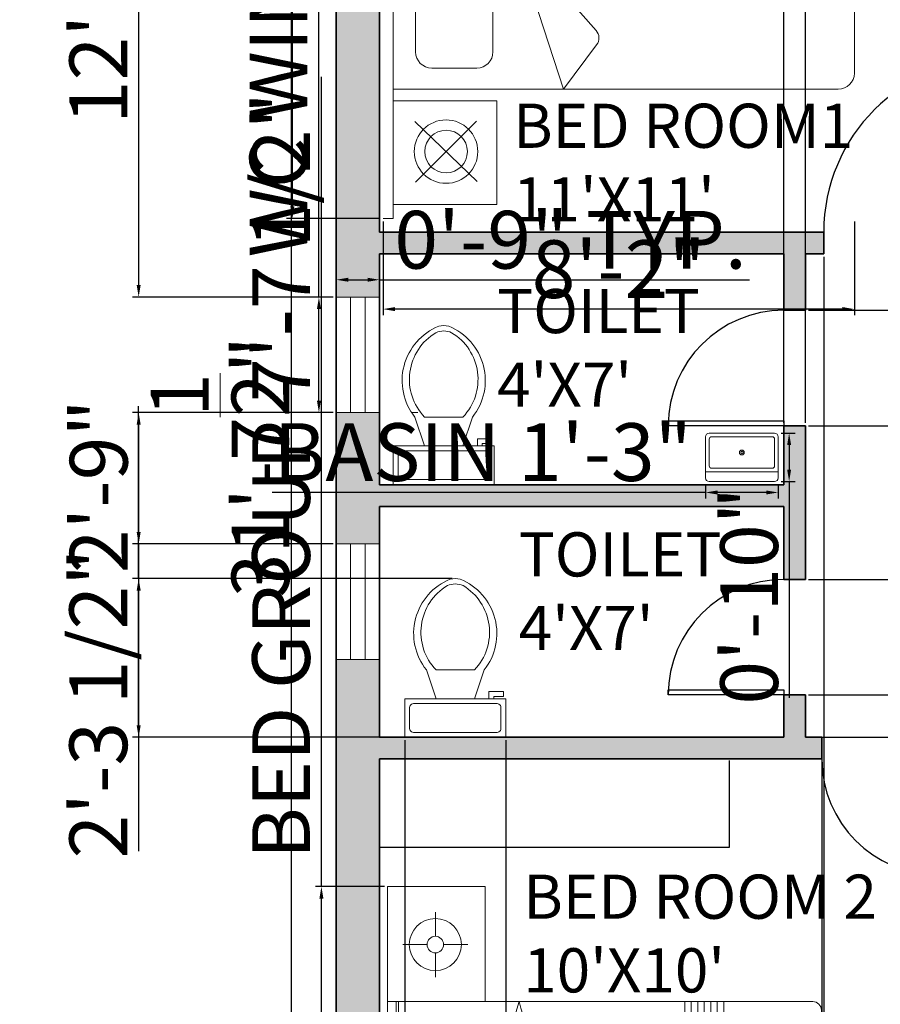
# Model space of a CAD drawing. Units: inches. Extents: x 1810 to 2254, y 313 to 1026.
# Tile 3 of 7: x 1810 to 1988, y 559 to 764. Entities that reach past the tile are written whole.
import ezdxf

# ---------------------------------------------------------------- set-up
doc = ezdxf.new("R2010")
doc.units = ezdxf.units.IN
for name, color, linetype, lineweight in [('A-ANNO-DIMS', 2, 'Continuous', 18), ('A-AREA-IDEN', 7, 'Continuous', 25), ('A-DOOR', 4, 'Continuous', 25), ('A-FLOR-CASE', 8, 'Continuous', 25), ('A-FLOR-FIXT', 9, 'Continuous', 18), ('A-FURN', 8, 'Continuous', 18), ('A-GLAZ', 4, 'Continuous', 18), ('A-WALL', 7, 'Continuous', 35)]:
    doc.layers.add(name, color=color, linetype=linetype, lineweight=lineweight)
doc.layers.add('A-WALL-PATT', color=252, linetype='Continuous', lineweight=13, true_color=0x939598)
doc.styles.add('ATTR', font='romans.shx', dxfattribs={"width": 0.8, "height": 1.075})
doc.styles.get("Standard").update_dxf_attribs({"font": 'arial.ttf'})
doc.dimstyles.new('ISO-25', dxfattribs={"dimtxt": 12, "dimasz": 2.5, "dimexe": 1.25, "dimexo": 0.625, "dimtad": 1, "dimdec": 1, "dimlunit": 4, "dimtxsty": 'Standard', "dimcen": 2.5, "dimadec": 0, "dimazin": 0, "dimtfac": 1, "dimtdec": 1, "dimtmove": 0, "dimatfit": 3, "dimfxl": 1, "dimarcsym": 0})

# ---------------------------------------------------------------- blocks, each defined once
blk = doc.blocks.new('A$C5C1F5B49')
for p, q in [((0, 2), (0, 2.0434)), ((2.6204, 1.9984), (2.6204, 2.0434)), ((0, 2), (2.6204, 2)), ((0.5102, 2), (0.0602, 2)), ((0.0602, 2), (0.0602, 1.55)), ((0.5102, 1.55), (0.5102, 2)), ((0.5602, 2), (0.5602, 0.07)), ((2.0602, 2), (0.5602, 2)), ((2.0602, 0.07), (2.0602, 2)), ((2.5602, 2), (2.1102, 2)), ((2.1102, 2), (2.1102, 1.55)), ((2.5602, 1.55), (2.5602, 2)), ((0.1574, 1.9028), (0.4225, 1.6377)), ((0.1602, 1.635), (0.4197, 1.9056)), ((1.2033, 1.9024), (0.7221, 1.9024)), ((1.919, 1.9024), (1.4378, 1.9024)), ((2.2074, 1.9028), (2.4725, 1.6377)), ((2.2102, 1.635), (2.4697, 1.9056)), ((0.6521, 1.8324), (0.6521, 1.6369)), ((1.2733, 1.6369), (1.2733, 1.8324)), ((1.3678, 1.8324), (1.3678, 1.6369)), ((1.989, 1.6369), (1.989, 1.8324)), ((0.0602, 1.55), (0.5102, 1.55)), ((0.7221, 1.5669), (1.2033, 1.5669)), ((1.4378, 1.5669), (1.919, 1.5669)), ((2.1102, 1.55), (2.5602, 1.55)), ((0.5602, 1.2611), (1.2132, 1.4737)), ((1.2066, 1.4637), (0.8154, 1.12)), ((1.3997, 1.4761), (1.2396, 1.4761)), ((1.3997, 1.4761), (1.805, 1.12)), ((2.0602, 1.2611), (1.3997, 1.4761)), ((0.7525, 1.1175), (0.5602, 1.2611)), ((1.868, 1.1175), (2.0602, 1.2611)), ((0.6302, 0), (1.9902, 0))]:
    blk.add_line(p, q)
for centre, radius in [((0.2899, 1.7703), 0.1375), ((2.3399, 1.7703), 0.1375), ((0.2899, 1.7703), 0.0925), ((2.3399, 1.7703), 0.0925)]:
    blk.add_circle(centre, radius)
for centre, radius, start, end in [((0.7221, 1.8324), 0.07, 90, 180), ((1.2033, 1.8324), 0.07, 0, 90), ((1.4378, 1.8324), 0.07, 90, 180), ((1.919, 1.8324), 0.07, 0, 90), ((0.7221, 1.6369), 0.07, 180, 270), ((1.2033, 1.6369), 0.07, 270, 0), ((1.4378, 1.6369), 0.07, 180, 270), ((1.919, 1.6369), 0.07, 270, 0), ((1.2396, 1.4261), 0.05, 90, 131.3042), ((1.2287, 1.4261), 0.05, 90, 108.034), ((0.7824, 1.1575), 0.05, 233.2421, 311.3042), ((1.838, 1.1575), 0.05, 228.6958, 306.7579), ((0.6302, 0.07), 0.07, 180, 270), ((1.9902, 0.07), 0.07, 270, 0)]:
    blk.add_arc(centre, radius, start, end)
blk = doc.blocks.new('A$C50CC761E')
for p, q in [((0, 2), (0, 0.04)), ((0, 2), (1.5, 2)), ((1.5, 2), (1.5, 0.04)), ((0, 1.96), (1.5, 1.96)), ((0, 1.95), (1.5, 1.95)), ((0, 0.63), (1.5, 0.63)), ((0, 0.6), (1.5, 0.6)), ((0, 0.57), (1.5, 0.57)), ((0, 0.54), (1.5, 0.54)), ((0, 0.51), (1.5, 0.51)), ((0, 0.48), (1.5, 0.48)), ((0, 0.45), (1.5, 0.45)), ((1.46, 0), (0.04, 0))]:
    blk.add_line(p, q)
at = {"ltscale": 250}
for p, q in [((1.5, 2), (2.0303, 2)), ((2.0303, 2), (2.0303, 1.5501)), ((1.763, 1.8176), (1.763, 1.9295)), ((1.613, 1.7795), (1.7249, 1.7795)), ((1.8011, 1.7795), (1.913, 1.7795)), ((1.763, 1.6295), (1.763, 1.7414)), ((1.5, 1.5501), (2.0303, 1.5501))]:
    blk.add_line(p, q, dxfattribs=at)
for radius in [0.12, 0.0381]:
    blk.add_circle((1.763, 1.7795), radius, dxfattribs=at)
for centre, radius, start, end in [((0.3894, 5.1577), 3.2899, 265.4501, 274.5499), ((-0.4158, 1.744), 0.5605, 346.15, 13.85), ((0.1321, 1.5916), 0.3789, 4.7708, 46.8165), ((0.1321, 1.5916), 0.4089, 4.1373, 42.5614), ((0.1321, 1.5916), 0.4389, 3.5318, 39.1874), ((0.1321, 1.5916), 0.4689, 2.9489, 36.4321), ((1.1324, 1.744), 0.5004, 164.4468, 195.5532), ((1.1357, 5.1577), 3.2899, 265.4501, 274.5499), ((0.3306, 1.744), 0.5605, 346.15, 13.85), ((0.8784, 1.5916), 0.3789, 4.7708, 46.8165), ((0.8784, 1.5916), 0.4089, 4.1373, 42.5614), ((0.8784, 1.5916), 0.4389, 3.5318, 39.1874), ((0.8784, 1.5916), 0.4689, 2.9489, 36.4321), ((1.8788, 1.744), 0.5004, 164.4468, 195.5532), ((0.3894, -0.4129), 2.0395, 82.6483, 97.3517), ((1.1357, -0.4129), 2.0395, 82.6483, 97.3517), ((1.0573, -0.0269), 1.4879, 72.6898, 135.2822), ((1.6044, 0.9359), 0.4695, 102.8515, 161.769), ((0.6316, 0.0846), 1.1287, 62.1724, 124.0295), ((0.04, 0.04), 0.04, 180, 270), ((1.46, 0.04), 0.04, 270, 0)]:
    blk.add_arc(centre, radius, start, end)
blk = doc.blocks.new('*U4')
for p, q in [((9.5, -6), (9.5, -2)), ((-8, -8.5), (-8, -8)), ((-7, -8), (-7, -9.5)), ((-4, -8), (-6, -14)), ((4, -8), (6, -14)), ((-10, -8.5), (-8, -8.5)), ((-10, -9.5), (-10, -8.5)), ((-7, -9.5), (-10, -9.5)), ((4, -14), (-4, -14))]:
    blk.add_line(p, q)
blk.add_lwpolyline([(10.5, -8), (10.5, 0), (-10.5, 0), (-10.5, -8)], close=True)
for points in [[(-9.5, -2), (-9.5, -6)], [(8.5, -1), (-8.5, -1)], [(-8.5, -7), (8.5, -7)]]:
    blk.add_lwpolyline(points)
for centre, radius, start, end in [((-8.62, -1.88), 0.884, 81.8699, 188.1301), ((8.62, -1.88), 0.884, 351.8699, 98.1301), ((-8.62, -6.12), 0.884, 171.8699, 278.1301), ((8.62, -6.12), 0.884, 261.8699, 8.1301), ((3.52, -21.58), 12.17, 141.4691, 247.9714), ((4.2, -21.82), 11.33, 136.3677, 238.9468), ((-3.52, -21.58), 12.17, 292.0284, 38.5307), ((-4.2, -21.82), 11.33, 301.053, 43.6321), ((0, -27.88), 4, 245.7318, 294.2682), ((0, -29), 4, 254.8605, 285.1395)]:
    blk.add_arc(centre, radius, start, end)
blk = doc.blocks.new("30'' Sink Single PV")
blk.add_line((-15, -3.999996), (15, -3.999996))
for points in [[(-13.5, 0), (13.5, 0)], [(-15, -18.499996), (-15, -1.5)], [(15, -1.5), (15, -18.499996)], [(-13.5, -17.499996), (-13.5, -6.499996)], [(-12.5, -5.499996), (12.5, -5.499996)], [(13.5, -6.499996), (13.5, -17.499996)], [(13.5, -19.999996), (-13.5, -19.999996)], [(12.5, -18.499996), (-12.5, -18.499996)]]:
    blk.add_lwpolyline(points)
for radius in [1, 0.5]:
    blk.add_circle((0, -11.999996), radius)
for centre, radius, start, end in [((-13.5, -1.5), 1.5, 90, 180), ((13.5, -1.5), 1.5, 0, 90), ((-12.5, -6.499996), 1, 90, 180), ((12.5, -6.499996), 1, 0, 90), ((-13.5, -18.499996), 1.5, 180, 270), ((-12.5, -17.499996), 1, 180, 270), ((12.5, -17.499996), 1, 270, 0), ((13.5, -18.499996), 1.5, 270, 0)]:
    blk.add_arc(centre, radius, start, end)
at = {"style": 'ATTR', "width": 0.8, "flags": 9}
blk.add_attdef('ESTCODE', (0, 0), '', height=0.006, dxfattribs=at)
blk = doc.blocks.new('*U17')
for p, q in [((0, 0), (0, -4)), ((-40, 0), (-40, -4))]:
    blk.add_line(p, q)
blk.add_lwpolyline([(0, 0), (0, 40), (-1.75, 40), (-1.75, 0)], close=True)
blk.add_arc((0, 0), 40, 90, 180)
blk = doc.blocks.new('*U16')
for p, q in [((0, 0), (0, -6)), ((40, 0), (40, -6))]:
    blk.add_line(p, q)
blk.add_lwpolyline([(0, 0), (0, 40), (1.75, 40), (1.75, 0)], close=True)
blk.add_arc((0, 0), 40, 0, 90)
blk = doc.blocks.new('*D25')
at = {"layer": 'A-ANNO-DIMS', "color": 0, "lineweight": -2, "transparency": 16777216}
for p, q in [((1874.74, 860.61), (1864.75, 860.61)), ((1866, 858.11), (1866, 483.61)), ((1874.74, 481.11), (1864.75, 481.11))]:
    blk.add_line(p, q, dxfattribs=at)
at = {"layer": 'A-ANNO-DIMS', "color": 0, "transparency": 16777216}
for points in [[(1865.58, 858.11), (1866.42, 858.11), (1866, 860.61)], [(1865.58, 483.61), (1866.42, 483.61), (1866, 481.11)]]:
    blk.add_solid(points, dxfattribs=at)
at = {"layer": 'Defpoints', "color": 0, "transparency": 16777216}
for p in [(1875.36, 860.61), (1866, 481.11), (1875.36, 481.11)]:
    blk.add_point(p, dxfattribs=at)
at = {"layer": 'A-ANNO-DIMS', "color": 0, "transparency": 16777216, "insert": (1851.22, 670.86), "char_height": 12, "attachment_point": 5, "rotation": 90}
blk.add_mtext('31\'-7{\\H1x;\\S1/2;}"', dxfattribs=at)
blk = doc.blocks.new('WIN-24IN-WALL9')
for p, q in [((9, 24), (0, 24)), ((3, 24), (3, 0)), ((6, 24), (6, 0)), ((9, 0), (0, 0))]:
    blk.add_line(p, q)
blk = doc.blocks.new('*D34')
at = {"layer": 'A-ANNO-DIMS', "color": 0, "lineweight": -2, "transparency": 16777216}
for p, q in [((1871.76, 706.11), (1871.76, 894.3)), ((1874.74, 706.11), (1870.51, 706.11)), ((1871.76, 684.61), (1871.76, 703.61)), ((1874.74, 682.11), (1870.51, 682.11))]:
    blk.add_line(p, q, dxfattribs=at)
at = {"layer": 'A-ANNO-DIMS', "color": 0, "transparency": 16777216}
for points in [[(1871.35, 703.61), (1872.18, 703.61), (1871.76, 706.11)], [(1871.35, 684.61), (1872.18, 684.61), (1871.76, 682.11)]]:
    blk.add_solid(points, dxfattribs=at)
at = {"layer": 'Defpoints', "color": 0, "transparency": 16777216}
for p in [(1871.76, 706.11), (1875.36, 706.11), (1875.36, 682.11)]:
    blk.add_point(p, dxfattribs=at)
at = {"layer": 'A-ANNO-DIMS', "color": 0, "transparency": 16777216, "insert": (1864.93, 801.46), "char_height": 12, "attachment_point": 5, "rotation": 90}
blk.add_mtext('WC WINDOW 2\'-0" TYP.', dxfattribs=at)
blk = doc.blocks.new('*D35')
at = {"layer": 'A-ANNO-DIMS', "color": 0, "lineweight": -2, "transparency": 16777216}
for p, q in [((1875.36, 706.74), (1875.36, 710.96)), ((1884.36, 706.74), (1884.36, 710.96)), ((1877.86, 709.71), (1881.86, 709.71)), ((1884.36, 709.71), (1961.26, 709.71))]:
    blk.add_line(p, q, dxfattribs=at)
at = {"layer": 'A-ANNO-DIMS', "color": 0, "transparency": 16777216}
for points in [[(1877.86, 710.13), (1877.86, 709.3), (1875.36, 709.71)], [(1881.86, 710.13), (1881.86, 709.3), (1884.36, 709.71)]]:
    blk.add_solid(points, dxfattribs=at)
at = {"layer": 'Defpoints', "color": 0, "transparency": 16777216}
for p in [(1884.36, 709.71), (1875.36, 706.11), (1884.36, 706.11)]:
    blk.add_point(p, dxfattribs=at)
at = {"layer": 'A-ANNO-DIMS', "color": 0, "transparency": 16777216, "insert": (1924.06, 716.47), "char_height": 12, "attachment_point": 5}
blk.add_mtext('0\'-9" TYP.', dxfattribs=at)
blk = doc.blocks.new('*D36')
at = {"layer": 'A-ANNO-DIMS', "color": 0, "lineweight": -2, "transparency": 16777216}
for p, q in [((1866.25, 848.07), (1866.25, 1025.73)), ((1884.47, 848.07), (1865, 848.07)), ((1866.25, 724.95), (1866.25, 845.57)), ((1884.47, 722.45), (1865, 722.45))]:
    blk.add_line(p, q, dxfattribs=at)
at = {"layer": 'A-ANNO-DIMS', "color": 0, "transparency": 16777216}
for points in [[(1865.83, 845.57), (1866.66, 845.57), (1866.25, 848.07)], [(1865.83, 724.95), (1866.66, 724.95), (1866.25, 722.45)]]:
    blk.add_solid(points, dxfattribs=at)
at = {"layer": 'Defpoints', "color": 0, "transparency": 16777216}
for p in [(1866.25, 848.07), (1885.09, 848.07), (1885.09, 722.45)]:
    blk.add_point(p, dxfattribs=at)
at = {"layer": 'A-ANNO-DIMS', "color": 0, "transparency": 16777216, "insert": (1859.41, 938.15), "char_height": 12, "attachment_point": 5, "rotation": 90}
blk.add_mtext('BED GROUP 10\'-5 1/2"', dxfattribs=at)
blk = doc.blocks.new('*D37')
at = {"layer": 'A-ANNO-DIMS', "color": 0, "lineweight": -2, "transparency": 16777216}
for p, q in [((1885.09, 721.83), (1885.09, 702.36)), ((1983.05, 721.83), (1983.05, 702.36)), ((1980.55, 703.61), (1887.59, 703.61))]:
    blk.add_line(p, q, dxfattribs=at)
at = {"layer": 'A-ANNO-DIMS', "color": 0, "transparency": 16777216}
for points in [[(1887.59, 704.03), (1887.59, 703.19), (1885.09, 703.61)], [(1980.55, 704.03), (1980.55, 703.19), (1983.05, 703.61)]]:
    blk.add_solid(points, dxfattribs=at)
at = {"layer": 'Defpoints', "color": 0, "transparency": 16777216}
for p in [(1885.09, 722.45), (1983.05, 722.45), (1885.09, 703.61)]:
    blk.add_point(p, dxfattribs=at)
at = {"layer": 'A-ANNO-DIMS', "color": 0, "transparency": 16777216, "insert": (1934.07, 710.36), "char_height": 12, "attachment_point": 5}
blk.add_mtext('8\'-2"', dxfattribs=at)
blk = doc.blocks.new('*D38')
at = {"layer": 'A-ANNO-DIMS', "color": 0, "lineweight": -2, "transparency": 16777216}
for p, q in [((1872.28, 583.59), (1872.28, 751.92)), ((1885.39, 583.59), (1871.03, 583.59)), ((1872.28, 494.52), (1872.28, 581.09)), ((1885.39, 492.02), (1871.03, 492.02))]:
    blk.add_line(p, q, dxfattribs=at)
at = {"layer": 'A-ANNO-DIMS', "color": 0, "transparency": 16777216}
for points in [[(1871.87, 581.09), (1872.7, 581.09), (1872.28, 583.59)], [(1871.87, 494.52), (1872.7, 494.52), (1872.28, 492.02)]]:
    blk.add_solid(points, dxfattribs=at)
at = {"layer": 'Defpoints', "color": 0, "transparency": 16777216}
for p in [(1872.28, 583.59), (1886.02, 583.59), (1886.02, 492.02)]:
    blk.add_point(p, dxfattribs=at)
at = {"layer": 'A-ANNO-DIMS', "color": 0, "transparency": 16777216, "insert": (1865.45, 669.01), "char_height": 12, "attachment_point": 5, "rotation": 90}
blk.add_mtext('BED GROUP 7\'-7 1/2"', dxfattribs=at)
blk = doc.blocks.new('*D48')
at = {"layer": 'A-ANNO-DIMS', "color": 0, "lineweight": -2, "transparency": 16777216}
for p, q in [((1952.12, 665.5), (1862.04, 665.5)), ((1952.12, 667.14), (1952.12, 664.25)), ((1964.72, 665.5), (1954.62, 665.5)), ((1967.22, 667.14), (1967.22, 664.25))]:
    blk.add_line(p, q, dxfattribs=at)
at = {"layer": 'A-ANNO-DIMS', "color": 0, "transparency": 16777216}
for points in [[(1954.62, 665.91), (1954.62, 665.08), (1952.12, 665.5)], [(1964.72, 665.91), (1964.72, 665.08), (1967.22, 665.5)]]:
    blk.add_solid(points, dxfattribs=at)
at = {"layer": 'Defpoints', "color": 0, "transparency": 16777216}
for p in [(1952.12, 667.76), (1967.22, 667.76), (1952.12, 665.5)]:
    blk.add_point(p, dxfattribs=at)
at = {"layer": 'A-ANNO-DIMS', "color": 0, "transparency": 16777216, "insert": (1905.83, 672.33), "char_height": 12, "attachment_point": 5}
blk.add_mtext('BASIN 1\'-3"', dxfattribs=at)
blk = doc.blocks.new('*D49')
at = {"layer": 'A-ANNO-DIMS', "color": 0, "lineweight": -2, "transparency": 16777216}
for p, q in [((1967.85, 677.83), (1970.74, 677.83)), ((1969.49, 675.33), (1969.49, 670.26)), ((1967.85, 667.76), (1970.74, 667.76)), ((1969.49, 667.76), (1969.49, 622.79))]:
    blk.add_line(p, q, dxfattribs=at)
at = {"layer": 'A-ANNO-DIMS', "color": 0, "transparency": 16777216}
for points in [[(1969.07, 675.33), (1969.9, 675.33), (1969.49, 677.83)], [(1969.07, 670.26), (1969.9, 670.26), (1969.49, 667.76)]]:
    blk.add_solid(points, dxfattribs=at)
at = {"layer": 'Defpoints', "color": 0, "transparency": 16777216}
for p in [(1967.22, 677.83), (1967.22, 667.76), (1969.49, 667.76)]:
    blk.add_point(p, dxfattribs=at)
at = {"layer": 'A-ANNO-DIMS', "color": 0, "transparency": 16777216, "insert": (1962.73, 644.02), "char_height": 12, "attachment_point": 5, "rotation": 90}
blk.add_mtext('0\'-10"', dxfattribs=at)
blk = doc.blocks.new('*D55')
at = {"layer": 'A-ANNO-DIMS', "color": 0, "lineweight": -2, "transparency": 16777216}
for p, q in [((1874.74, 860.61), (1833.05, 860.61)), ((1834.3, 858.11), (1834.3, 708.61)), ((1874.74, 706.11), (1833.05, 706.11))]:
    blk.add_line(p, q, dxfattribs=at)
at = {"layer": 'A-ANNO-DIMS', "color": 0, "transparency": 16777216}
for points in [[(1833.89, 858.11), (1834.72, 858.11), (1834.3, 860.61)], [(1833.89, 708.61), (1834.72, 708.61), (1834.3, 706.11)]]:
    blk.add_solid(points, dxfattribs=at)
at = {"layer": 'Defpoints', "color": 0, "transparency": 16777216}
for p in [(1875.36, 860.61), (1834.3, 706.11), (1875.36, 706.11)]:
    blk.add_point(p, dxfattribs=at)
at = {"layer": 'A-ANNO-DIMS', "color": 0, "transparency": 16777216, "insert": (1827.47, 783.36), "char_height": 12, "attachment_point": 5, "rotation": 90}
blk.add_mtext('12\'-10 1/2"', dxfattribs=at)
blk = doc.blocks.new('*D56')
at = {"layer": 'A-ANNO-DIMS', "color": 0, "lineweight": -2, "transparency": 16777216}
for p, q in [((1874.74, 682.11), (1833.05, 682.11)), ((1834.3, 679.61), (1834.3, 657.29)), ((1874.74, 654.79), (1833.05, 654.79)), ((1834.3, 654.79), (1834.3, 590.97))]:
    blk.add_line(p, q, dxfattribs=at)
at = {"layer": 'A-ANNO-DIMS', "color": 0, "transparency": 16777216}
for points in [[(1833.89, 679.61), (1834.72, 679.61), (1834.3, 682.11)], [(1833.89, 657.29), (1834.72, 657.29), (1834.3, 654.79)]]:
    blk.add_solid(points, dxfattribs=at)
at = {"layer": 'Defpoints', "color": 0, "transparency": 16777216}
for p in [(1875.36, 682.11), (1834.3, 654.79), (1875.36, 654.79)]:
    blk.add_point(p, dxfattribs=at)
at = {"layer": 'A-ANNO-DIMS', "color": 0, "transparency": 16777216, "insert": (1827.47, 621.63), "char_height": 12, "attachment_point": 5, "rotation": 90}
blk.add_mtext('2\'-3 1/2"', dxfattribs=at)
blk = doc.blocks.new('*D62')
at = {"layer": 'A-ANNO-DIMS', "color": 0, "lineweight": -2, "transparency": 16777216}
for p, q in [((2169.76, 703.36), (2169.76, 739.21)), ((1973.49, 703.36), (2171.01, 703.36)), ((2169.76, 681.86), (2169.76, 700.86)), ((1973.49, 679.36), (2171.01, 679.36))]:
    blk.add_line(p, q, dxfattribs=at)
at = {"layer": 'A-ANNO-DIMS', "color": 0, "transparency": 16777216}
for points in [[(2169.35, 700.86), (2170.18, 700.86), (2169.76, 703.36)], [(2169.35, 681.86), (2170.18, 681.86), (2169.76, 679.36)]]:
    blk.add_solid(points, dxfattribs=at)
at = {"layer": 'Defpoints', "color": 0, "transparency": 16777216}
for p in [(1972.86, 703.36), (2169.76, 703.36), (1972.86, 679.36)]:
    blk.add_point(p, dxfattribs=at)
at = {"layer": 'A-ANNO-DIMS', "color": 0, "transparency": 16777216, "insert": (2163.01, 722.54), "char_height": 12, "attachment_point": 5, "rotation": 90}
blk.add_mtext('2\'-0"', dxfattribs=at)
blk = doc.blocks.new('*D63')
at = {"layer": 'A-ANNO-DIMS', "color": 0, "lineweight": -2, "transparency": 16777216}
for p, q in [((2169.76, 679.36), (2169.76, 715.21)), ((1973.49, 679.36), (2171.01, 679.36)), ((2169.76, 649.92), (2169.76, 676.86)), ((1973.49, 647.42), (2171.01, 647.42))]:
    blk.add_line(p, q, dxfattribs=at)
at = {"layer": 'A-ANNO-DIMS', "color": 0, "transparency": 16777216}
for points in [[(2169.35, 676.86), (2170.18, 676.86), (2169.76, 679.36)], [(2169.35, 649.92), (2170.18, 649.92), (2169.76, 647.42)]]:
    blk.add_solid(points, dxfattribs=at)
at = {"layer": 'Defpoints', "color": 0, "transparency": 16777216}
for p in [(1972.86, 679.36), (2169.76, 679.36), (1972.86, 647.42)]:
    blk.add_point(p, dxfattribs=at)
at = {"layer": 'A-ANNO-DIMS', "color": 0, "transparency": 16777216, "insert": (2163.01, 698.54), "char_height": 12, "attachment_point": 5, "rotation": 90}
blk.add_mtext('2\'-8"', dxfattribs=at)
blk = doc.blocks.new('*D64')
at = {"layer": 'A-ANNO-DIMS', "color": 0, "lineweight": -2, "transparency": 16777216}
for p, q in [((2169.76, 623.42), (2169.76, 659.07)), ((1973.49, 623.42), (2171.01, 623.42)), ((2169.76, 617.11), (2169.76, 620.92)), ((1973.49, 614.61), (2171.01, 614.61))]:
    blk.add_line(p, q, dxfattribs=at)
at = {"layer": 'A-ANNO-DIMS', "color": 0, "transparency": 16777216}
for points in [[(2169.35, 620.92), (2170.18, 620.92), (2169.76, 623.42)], [(2169.35, 617.11), (2170.18, 617.11), (2169.76, 614.61)]]:
    blk.add_solid(points, dxfattribs=at)
at = {"layer": 'Defpoints', "color": 0, "transparency": 16777216}
for p in [(1972.86, 623.42), (2169.76, 623.42), (1972.86, 614.61)]:
    blk.add_point(p, dxfattribs=at)
at = {"layer": 'A-ANNO-DIMS', "color": 0, "transparency": 16777216, "insert": (2163.01, 642.49), "char_height": 12, "attachment_point": 5, "rotation": 90}
blk.add_mtext('0\'-9"', dxfattribs=at)
blk = doc.blocks.new('*D65')
at = {"layer": 'A-ANNO-DIMS', "color": 0, "lineweight": -2, "transparency": 16777216}
for p, q in [((1965.86, 891.01), (1963.36, 891.01)), ((1968.36, 679.98), (1968.36, 892.26)), ((1968.36, 891.01), (1972.86, 891.01)), ((1972.86, 679.98), (1972.86, 892.26)), ((1975.36, 891.01), (2038.97, 891.01))]:
    blk.add_line(p, q, dxfattribs=at)
at = {"layer": 'A-ANNO-DIMS', "color": 0, "transparency": 16777216}
for points in [[(1965.86, 891.43), (1965.86, 890.6), (1968.36, 891.01)], [(1975.36, 891.43), (1975.36, 890.6), (1972.86, 891.01)]]:
    blk.add_solid(points, dxfattribs=at)
at = {"layer": 'Defpoints', "color": 0, "transparency": 16777216}
for p in [(1972.86, 891.01), (1968.36, 679.36), (1972.86, 679.36)]:
    blk.add_point(p, dxfattribs=at)
at = {"layer": 'A-ANNO-DIMS', "color": 0, "transparency": 16777216, "insert": (2008.42, 897.84), "char_height": 12, "attachment_point": 5}
blk.add_mtext('0\'-4 1/2"', dxfattribs=at)
blk = doc.blocks.new('*D66')
at = {"layer": 'A-ANNO-DIMS', "color": 0, "lineweight": -2, "transparency": 16777216}
for p, q in [((1976.27, 609.49), (1976.27, 323.71)), ((2000.27, 609.49), (2000.27, 323.71)), ((1978.77, 324.96), (1997.77, 324.96)), ((2000.27, 324.96), (2036.12, 324.96))]:
    blk.add_line(p, q, dxfattribs=at)
at = {"layer": 'A-ANNO-DIMS', "color": 0, "transparency": 16777216}
for points in [[(1978.77, 325.38), (1978.77, 324.55), (1976.27, 324.96)], [(1997.77, 325.38), (1997.77, 324.55), (2000.27, 324.96)]]:
    blk.add_solid(points, dxfattribs=at)
at = {"layer": 'Defpoints', "color": 0, "transparency": 16777216}
for p in [(1976.27, 610.11), (2000.27, 610.11), (2000.27, 324.96)]:
    blk.add_point(p, dxfattribs=at)
at = {"layer": 'A-ANNO-DIMS', "color": 0, "transparency": 16777216, "insert": (2019.45, 331.72), "char_height": 12, "attachment_point": 5}
blk.add_mtext('2\'-0"', dxfattribs=at)
blk = doc.blocks.new('*D67')
at = {"layer": 'A-ANNO-DIMS', "color": 0, "lineweight": -2, "transparency": 16777216}
for p, q in [((1976.68, 714.49), (1976.68, 323.71)), ((2012.68, 714.49), (2012.68, 323.71)), ((1979.18, 324.96), (2010.18, 324.96))]:
    blk.add_line(p, q, dxfattribs=at)
at = {"layer": 'A-ANNO-DIMS', "color": 0, "transparency": 16777216}
for points in [[(1979.18, 325.38), (1979.18, 324.55), (1976.68, 324.96)], [(2010.18, 325.38), (2010.18, 324.55), (2012.68, 324.96)]]:
    blk.add_solid(points, dxfattribs=at)
at = {"layer": 'Defpoints', "color": 0, "transparency": 16777216}
for p in [(1976.68, 715.11), (2012.68, 715.11), (2012.68, 324.96)]:
    blk.add_point(p, dxfattribs=at)
at = {"layer": 'A-ANNO-DIMS', "color": 0, "transparency": 16777216, "insert": (1994.68, 331.72), "char_height": 12, "attachment_point": 5}
blk.add_mtext('3\'-0"', dxfattribs=at)
blk = doc.blocks.new('*D72')
at = {"layer": 'A-ANNO-DIMS', "color": 0, "lineweight": -2, "transparency": 16777216}
for p, q in [((1889.6, 613.99), (1889.6, 323.71)), ((1910.6, 613.99), (1910.6, 323.71)), ((1892.1, 324.96), (1908.1, 324.96)), ((1910.6, 324.96), (1945.12, 324.96))]:
    blk.add_line(p, q, dxfattribs=at)
at = {"layer": 'A-ANNO-DIMS', "color": 0, "transparency": 16777216}
for points in [[(1892.1, 325.38), (1892.1, 324.55), (1889.6, 324.96)], [(1908.1, 325.38), (1908.1, 324.55), (1910.6, 324.96)]]:
    blk.add_solid(points, dxfattribs=at)
at = {"layer": 'Defpoints', "color": 0, "transparency": 16777216}
for p in [(1889.6, 614.61), (1910.6, 614.61), (1910.6, 324.96)]:
    blk.add_point(p, dxfattribs=at)
at = {"layer": 'A-ANNO-DIMS', "color": 0, "transparency": 16777216, "insert": (1929.11, 331.72), "char_height": 12, "attachment_point": 5}
blk.add_mtext('1\'-9"', dxfattribs=at)
blk = doc.blocks.new('*D73')
at = {"layer": 'A-ANNO-DIMS', "color": 0, "lineweight": -2, "transparency": 16777216}
for p, q in [((1834.3, 647.61), (1834.3, 683.47)), ((1899.48, 647.61), (1833.05, 647.61)), ((1834.3, 617.11), (1834.3, 645.11)), ((1888.98, 614.61), (1833.05, 614.61))]:
    blk.add_line(p, q, dxfattribs=at)
at = {"layer": 'A-ANNO-DIMS', "color": 0, "transparency": 16777216}
for points in [[(1833.89, 645.11), (1834.72, 645.11), (1834.3, 647.61)], [(1833.89, 617.11), (1834.72, 617.11), (1834.3, 614.61)]]:
    blk.add_solid(points, dxfattribs=at)
at = {"layer": 'Defpoints', "color": 0, "transparency": 16777216}
for p in [(1834.3, 647.61), (1900.1, 647.61), (1889.6, 614.61)]:
    blk.add_point(p, dxfattribs=at)
at = {"layer": 'A-ANNO-DIMS', "color": 0, "transparency": 16777216, "insert": (1827.55, 666.79), "char_height": 12, "attachment_point": 5, "rotation": 90}
blk.add_mtext('2\'-9"', dxfattribs=at)

msp = doc.modelspace()

# ---------------------------------------------------------------- hatches: boundary and pattern name
at = {"layer": 'A-WALL-PATT'}
h = msp.add_hatch(color=256, dxfattribs=at)
h.dxf.hatch_style = 1
h.paths.add_polyline_path([(1943.78, 860.61), (1875.36, 860.61), (1875.36, 706.11), (1884.36, 706.11), (1884.36, 715.11), (1968.36, 715.11), (1968.36, 703.36), (1971.96, 703.36), (1972.86, 703.36), (1972.86, 715.11), (1976.68, 715.11), (1976.68, 719.61), (1884.36, 719.61), (1884.36, 851.61), (1943.73, 851.61)])
h.paths.add_polyline_path([(2048.15, 860.61), (1979.78, 860.61), (1979.73, 851.61), (2016.36, 851.61), (2016.36, 719.61), (2012.68, 719.61), (2012.68, 716.01), (2012.68, 715.11), (2024.44, 715.11), (2024.44, 719.61), (2020.86, 719.61), (2020.86, 851.61), (2048.15, 851.61)])
h.paths.add_polyline_path([(2139.36, 860.61), (2084.15, 860.61), (2084.15, 851.61), (2130.36, 851.61), (2130.36, 719.61), (2060.44, 719.61), (2060.44, 716.01), (2060.44, 715.11), (2130.36, 715.11), (2130.36, 673.52), (2139.36, 673.52)])
h.paths.add_polyline_path([(1884.36, 682.11), (1875.36, 682.11), (1875.36, 654.79), (1884.36, 654.79), (1884.36, 662.61), (1968.36, 662.61), (1968.36, 647.42), (1971.96, 647.42), (1972.86, 647.42), (1972.86, 679.36), (1968.36, 679.36), (1968.36, 667.11), (1884.36, 667.11)])
h.paths.add_polyline_path([(1884.36, 610.11), (1972.86, 610.11), (1976.27, 610.11), (1976.27, 614.61), (1972.86, 614.61), (1972.86, 623.42), (1968.36, 623.42), (1968.36, 614.61), (1884.36, 614.61), (1884.36, 630.79), (1875.36, 630.79), (1875.36, 481.11), (1939.68, 481.11), (1939.68, 490.11), (1884.36, 490.11)])
h.paths.add_polyline_path([(2007.36, 518.61), (2038.86, 518.61), (2038.86, 494.59), (2043.36, 494.59), (2043.36, 518.61), (2070.36, 518.61), (2070.36, 523.11), (2007.36, 523.11), (2007.36, 614.61), (2000.27, 614.61), (2000.27, 610.11), (2003.36, 610.11), (2003.36, 490.11), (1975.68, 490.11), (1975.68, 481.11), (2007.36, 481.11)])
h.paths.add_polyline_path([(2139.36, 637.52), (2130.36, 637.52), (2130.36, 434.61), (2043.36, 434.61), (2043.36, 458.59), (2038.86, 458.59), (2038.86, 434.61), (2035.41, 434.61), (2035.41, 431.01), (2035.41, 425.61), (2139.36, 425.61)])

# ---------------------------------------------------------------- linework, layer by layer
at = {"layer": 'A-FLOR-CASE'}
for p, q in [((1957.11, 591.78), (1957.11, 609.78)), ((1884.36, 591.78), (1957.11, 591.78))]:
    msp.add_line(p, q, dxfattribs=at)
at = {"layer": 'A-GLAZ'}
for p, q in [((1892.33, 682.11), (1891.03, 682.11)), ((1892.78, 630.79), (1892.72, 630.79))]:
    msp.add_line(p, q, dxfattribs=at)
at = {"layer": 'A-WALL'}
for p, q in [((1875.36, 860.61), (1875.36, 481.11)), ((1884.36, 851.61), (1884.36, 719.61)), ((1884.36, 719.61), (1976.68, 719.61)), ((1976.68, 719.61), (1976.68, 715.11)), ((1884.36, 715.11), (1968.36, 715.11)), ((1884.36, 715.11), (1884.36, 667.11)), ((1968.36, 715.11), (1968.36, 703.36)), ((1972.86, 715.11), (1972.86, 703.36)), ((1972.86, 715.11), (1976.68, 715.11)), ((1968.36, 703.36), (1972.86, 703.36)), ((1968.36, 679.36), (1972.86, 679.36)), ((1968.36, 679.36), (1968.36, 667.11)), ((1972.86, 679.36), (1972.86, 647.42)), ((1884.36, 667.11), (1968.36, 667.11)), ((1884.36, 662.61), (1968.36, 662.61)), ((1884.36, 662.61), (1884.36, 614.61)), ((1968.36, 662.61), (1968.36, 647.42)), ((1968.36, 647.42), (1972.86, 647.42)), ((1968.36, 623.42), (1972.86, 623.42)), ((1968.36, 623.42), (1968.36, 614.61)), ((1972.86, 623.42), (1972.86, 614.61)), ((1884.36, 614.61), (1968.36, 614.61)), ((1976.27, 614.61), (1972.86, 614.61)), ((1976.27, 614.61), (1976.27, 610.11)), ((1884.36, 610.11), (1972.86, 610.11)), ((1884.36, 610.11), (1884.36, 490.11)), ((1976.27, 610.11), (1972.86, 610.11))]:
    msp.add_line(p, q, dxfattribs=at)

# ---------------------------------------------------------------- block references
at = {"layer": 'A-DOOR', "xscale": 0.8999999999999948, "yscale": 0.8999999999999948, "zscale": 0.8999999999999948}
msp.add_blockref('*U17', (2012.68, 719.61), dxfattribs=at)
at = {"layer": 'A-DOOR', "xscale": 0.6, "yscale": 0.6, "zscale": 0.6}
for p, rotation in [((1968.36, 679.36), 90.00000000000055), ((1968.36, 623.42), 90.00000000000055), ((2000.27, 610.11), 180)]:
    msp.add_blockref('*U16', p, dxfattribs=dict(at, rotation=rotation))
at = {"layer": 'A-FLOR-FIXT', "rotation": 180}
for p in [(1897.7, 667.18), (1900.1, 614.61)]:
    msp.add_blockref('*U4', p, dxfattribs=at)
at = {"layer": 'A-FLOR-FIXT', "xscale": 0.503213402023372, "yscale": 0.503213402023372, "zscale": 0.503213402023372, "rotation": 180}
msp.add_blockref("30'' Sink Single PV", (1959.67, 667.76), dxfattribs=at)
at = {"layer": 'A-FURN', "rotation": 90}
for name, p, xscale, yscale, zscale in [('A$C5C1F5B49', (1983.05, 722.45), 47.93842186149659, 47.93842186149659, 47.93842186149659), ('A$C50CC761E', (1976.21, 492.02), 45.09822183510779, 45.09822183510779, 45.09822183510779)]:
    msp.add_blockref(name, p, dxfattribs=dict(at, xscale=xscale, yscale=yscale, zscale=zscale))
at = {"layer": 'A-GLAZ'}
for p in [(1875.36, 682.11), (1875.36, 630.79)]:
    msp.add_blockref('WIN-24IN-WALL9', p, dxfattribs=at)

# ---------------------------------------------------------------- texts
at = {"layer": 'A-AREA-IDEN', "attachment_point": 1}
for s, width, insert, char_height in [("BED ROOM1 \\P11'X11'", 91.1081, (1912.12, 746.31), 9.181), ("TOILET\\P4'X7'", 11.8058, (1908.81, 707.79), 9.181), ("TOILET\\P4'X7'", 11.8058, (1913.28, 657.22), 9.181), ("BED ROOM 2 \\P10'X10'", 91.1081, (1914.23, 586.07), 9.1812)]:
    msp.add_mtext_dynamic_manual_height_columns(s, width=width, gutter_width=45.91, heights=[0], dxfattribs=dict(at, insert=insert, char_height=char_height))

# ---------------------------------------------------------------- dimensions: what is measured, and where the dimension line sits
at = {"layer": 'A-ANNO-DIMS'}
for base, p1, p2, angle, text, picture, middle in [((1866.25, 848.07), (1885.09, 722.45), (1885.09, 848.07), 90, 'BED GROUP <>', '*D36', (1859.41, 938.15)), ((1871.76, 706.11), (1875.36, 682.11), (1875.36, 706.11), 90, 'WC WINDOW <> TYP.', '*D34', (1864.93, 801.46)), ((1872.28, 583.59), (1886.02, 492.02), (1886.02, 583.59), 90, 'BED GROUP <>', '*D38', (1865.45, 669.01)), ((1952.12, 665.5), (1967.22, 667.76), (1952.12, 667.76), 180, 'BASIN <>', '*D48', (1905.83, 672.33))]:
    dim = msp.add_linear_dim(base=base, p1=p1, p2=p2, angle=angle, text=text, dimstyle='ISO-25', override={"dimdec": 1, "dimlfac": 1, "dimrnd": 0, "dimzin": 1, "dimdsep": 46, "dimlunit": 4, "dimfrac": 2}, dxfattribs=at)
    dim.commit()
    dim.dimension.update_dxf_attribs({"geometry": picture, "text_midpoint": middle})
for base, p1, p2, picture, middle in [((1972.86, 891.01), (1968.36, 679.36), (1972.86, 679.36), '*D65', (2008.42, 897.84)), ((2012.68, 324.96), (1976.68, 715.11), (2012.68, 715.11), '*D67', (1994.68, 331.72)), ((1910.6, 324.96), (1889.6, 614.61), (1910.6, 614.61), '*D72', (1929.11, 331.72)), ((2000.27, 324.96), (1976.27, 610.11), (2000.27, 610.11), '*D66', (2019.45, 331.72))]:
    dim = msp.add_linear_dim(base=base, p1=p1, p2=p2, dimstyle='ISO-25', override={"dimdec": 1, "dimlfac": 1, "dimrnd": 0, "dimzin": 1, "dimdsep": 46, "dimlunit": 4, "dimfrac": 2}, dxfattribs=at)
    dim.commit()
    dim.dimension.update_dxf_attribs({"geometry": picture, "text_midpoint": middle})
for base, p1, p2, angle, override, picture, middle in [((1834.3, 706.11), (1875.36, 860.61), (1875.36, 706.11), 90, {"dimdec": 1, "dimlfac": 1, "dimrnd": 0, "dimzin": 1, "dimdsep": 46, "dimlunit": 4, "dimfrac": 2}, '*D55', (1827.47, 783.36)), ((1866, 481.11), (1875.36, 860.61), (1875.36, 481.11), 90, {"dimclrd": 0, "dimclre": 0, "dimclrt": 0}, '*D25', (1851.22, 670.86)), ((2169.76, 703.36), (1972.86, 679.36), (1972.86, 703.36), 90, {"dimdec": 1, "dimlfac": 1, "dimrnd": 0, "dimzin": 1, "dimdsep": 46, "dimlunit": 4, "dimfrac": 2}, '*D62', (2163.01, 722.54)), ((1885.09, 703.61), (1983.05, 722.45), (1885.09, 722.45), 180, {"dimdec": 1, "dimlfac": 1, "dimrnd": 0, "dimzin": 1, "dimdsep": 46, "dimlunit": 4, "dimfrac": 2}, '*D37', (1934.07, 710.36)), ((2169.76, 679.36), (1972.86, 647.42), (1972.86, 679.36), 90, {"dimdec": 1, "dimlfac": 1, "dimrnd": 0, "dimzin": 1, "dimdsep": 46, "dimlunit": 4, "dimfrac": 2}, '*D63', (2163.01, 698.54)), ((1834.3, 647.61), (1889.6, 614.61), (1900.1, 647.61), 90, {"dimdec": 1, "dimlfac": 1, "dimrnd": 0, "dimzin": 1, "dimdsep": 46, "dimlunit": 4, "dimfrac": 2}, '*D73', (1827.55, 666.79)), ((1834.3, 654.79), (1875.36, 682.11), (1875.36, 654.79), 90, {"dimdec": 1, "dimlfac": 1, "dimrnd": 0, "dimzin": 1, "dimdsep": 46, "dimlunit": 4, "dimfrac": 2}, '*D56', (1827.47, 621.63)), ((1969.49, 667.76), (1967.22, 677.83), (1967.22, 667.76), 270, {"dimdec": 1, "dimlfac": 1, "dimrnd": 0, "dimzin": 1, "dimdsep": 46, "dimlunit": 4, "dimfrac": 2}, '*D49', (1962.73, 644.02)), ((2169.76, 623.42), (1972.86, 614.61), (1972.86, 623.42), 90, {"dimdec": 1, "dimlfac": 1, "dimrnd": 0, "dimzin": 1, "dimdsep": 46, "dimlunit": 4, "dimfrac": 2}, '*D64', (2163.01, 642.49))]:
    dim = msp.add_linear_dim(base=base, p1=p1, p2=p2, angle=angle, dimstyle='ISO-25', override=override, dxfattribs=at)
    dim.commit()
    dim.dimension.update_dxf_attribs({"geometry": picture, "text_midpoint": middle})
dim = msp.add_linear_dim(base=(1884.36, 709.71), p1=(1875.36, 706.11), p2=(1884.36, 706.11), text='<> TYP.', dimstyle='ISO-25', override={"dimdec": 1, "dimlfac": 1, "dimrnd": 0, "dimzin": 1, "dimdsep": 46, "dimlunit": 4, "dimfrac": 2}, dxfattribs=at)
dim.commit()
dim.dimension.update_dxf_attribs({"geometry": '*D35', "text_midpoint": (1924.06, 716.47)})

doc.saveas('drawing.dxf')
